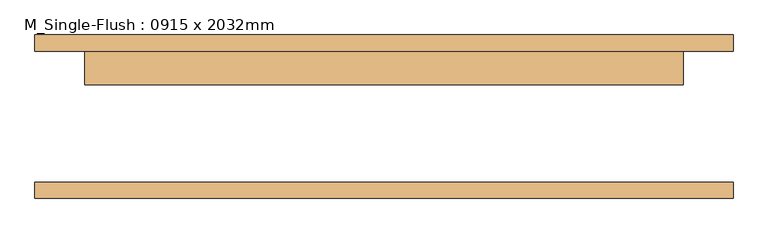
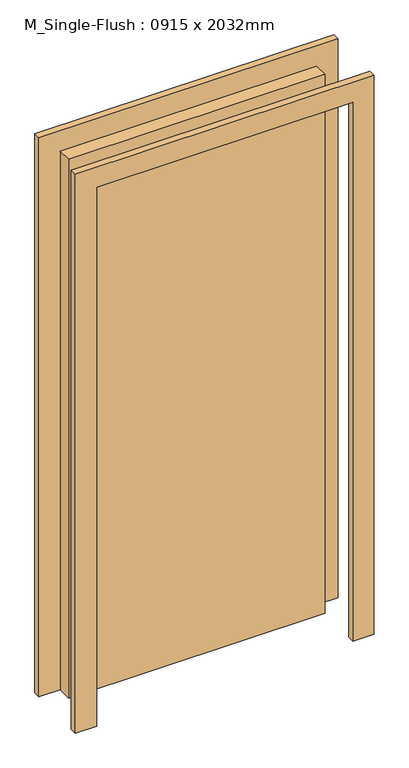
"""IFC4 building model written with IfcOpenShell, lengths in millimetres: door geometry, M_Single-Flush : 0915 x 2032mm."""

from ifc_helpers import new_model, si_unit, frame, origin, origin_with_axes, place, context, project, spatial, polyline, outline, extrude, source, transform, mapped, element, save


def m_single_flush_0915_x_2032mm_7267827e(model_context):
    return source(origin(), model_context, "Body", "SweptSolid", [
        extrude(outline(polyline([(2108.0, -533.5), (0.0, -533.5), (0.0, -457.5), (2032.0, -457.5), (2032.0, 457.5), (0.0, 457.5), (0.0, 533.5), (2108.0, 533.5), (2108.0, -533.5)])), frame((0.0, 100.0, 0.0), z_axis=(0.0, 1.0, 0.0), x_axis=(0.0, 0.0, 1.0)), (0.0, 0.0, 1.0), 25.0),
        extrude(outline(polyline([(2108.0, 533.5), (2108.0, -533.5), (0.0, -533.5), (0.0, -457.5), (2032.0, -457.5), (2032.0, 457.5), (0.0, 457.5), (0.0, 533.5), (2108.0, 533.5)])), frame((0.0, -125.0, 0.0), z_axis=(0.0, 1.0, 0.0), x_axis=(0.0, 0.0, 1.0)), (0.0, 0.0, 1.0), 25.0),
        extrude(outline(polyline([(457.5, 49.0), (-457.5, 49.0), (-457.5, 100.0), (457.5, 100.0), (457.5, 49.0)])), origin_with_axes(), (0.0, 0.0, 1.0), 2032.0),
    ])


if __name__ == "__main__":
    model = new_model("IFC4")
    model_context = context("Model", 3, world=origin())
    ifc_project = project(units=[si_unit("LENGTHUNIT", "METRE", prefix="MILLI")], contexts=[model_context])
    site = spatial("IfcSite", under=ifc_project)
    building = spatial("IfcBuilding", under=site)
    placement = place(None, origin())
    m_single_flush_0915_x_2032mm_shape = m_single_flush_0915_x_2032mm_7267827e(model_context)
    element("IfcDoor", 1, ObjectType="M_Single-Flush : 0915 x 2032mm", at=placement, inside=building, context=model_context, shape_type="MappedRepresentation", body=[
        mapped(m_single_flush_0915_x_2032mm_shape, transform((0.0, 0.0, 0.0), x_axis=(1.0, 0.0, 0.0), y_axis=(0.0, 1.0, 0.0), z_axis=(0.0, 0.0, 1.0))),
    ])
    save(model, "model.ifc")

# Revit data of these elements
# Type "M_Single-Flush : 0915 x 2032mm"
#   Type Mark = "20"
#   Thickness = 51 mm
#   Height = 2032 mm
#   Trim Projection Ext = 25 mm
#   Trim Projection Int = 25 mm
#   Trim Width = 76 mm
#   Width = 915 mm
#   Door Material = Door - Panel
#   Frame Material = Door - Frame
#   Function = (empty or 0)
#   Wall Closure = (empty or 0)
# Element 1 (IfcDoor, "M_Single-Flush : 0915 x 2032mm")
#   Materials on its faces: "Door - Frame", "Door - Panel"
# Materials
#   "Door - Panel": class "Wood", colour RGB 114 82 51, transparency 0
#   "Door - Frame": colour RGB 153 76 43, transparency 0
